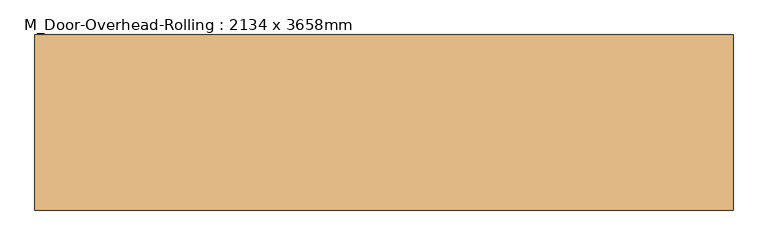
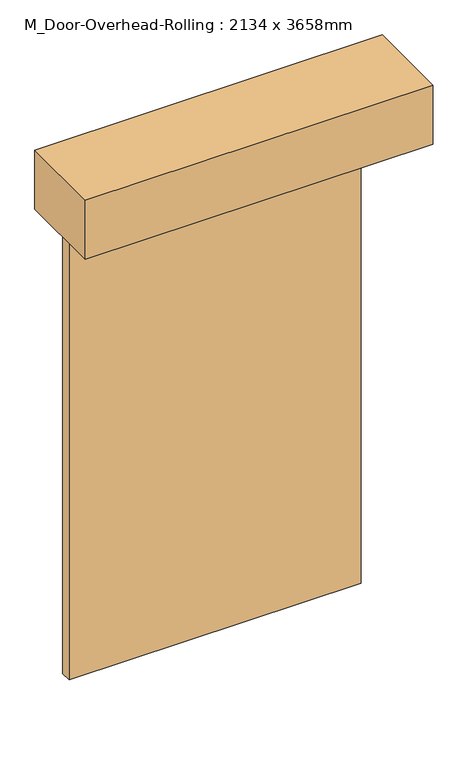
"""IFC4 building model written with IfcOpenShell, lengths in millimetres: door geometry, M_Door-Overhead-Rolling : 2134 x 3658mm."""

from ifc_helpers import new_model, si_unit, frame, origin, origin_with_axes, place, context, project, spatial, polyline, outline, extrude, source, transform, mapped, element, save


def m_door_overhead_rolling_2134_x_3658mm_be0fe279(model_context):
    return source(origin(), model_context, "Body", "SweptSolid", [
        extrude(outline(polyline([(1066.8, -114.3), (1066.8, -194.3), (-1066.8, -194.3), (-1066.8, -114.3), (1066.8, -114.3)])), origin_with_axes(), (0.0, 0.0, 1.0), 3657.6),
        extrude(outline(polyline([(1270.0, -753.1), (-1270.0, -753.1), (-1270.0, -114.3), (1270.0, -114.3), (1270.0, -753.1)])), frame((0.0, 0.0, 3657.6), z_axis=(0.0, 0.0, 1.0), x_axis=(1.0, 0.0, 0.0)), (0.0, 0.0, 1.0), 457.2),
    ])


if __name__ == "__main__":
    model = new_model("IFC4")
    model_context = context("Model", 3, world=origin())
    ifc_project = project(units=[si_unit("LENGTHUNIT", "METRE", prefix="MILLI")], contexts=[model_context])
    site = spatial("IfcSite", under=ifc_project)
    building = spatial("IfcBuilding", under=site)
    placement = place(None, origin())
    m_door_overhead_rolling_2134_x_3658mm_shape = m_door_overhead_rolling_2134_x_3658mm_be0fe279(model_context)
    element("IfcDoor", 1, ObjectType="M_Door-Overhead-Rolling : 2134 x 3658mm", at=placement, inside=building, context=model_context, shape_type="MappedRepresentation", body=[
        mapped(m_door_overhead_rolling_2134_x_3658mm_shape, transform((0.0, 0.0, 0.0), x_axis=(1.0, 0.0, 0.0), y_axis=(0.0, 1.0, 0.0), z_axis=(0.0, 0.0, 1.0))),
    ])
    save(model, "model.ifc")

# Revit data of these elements
# Type "M_Door-Overhead-Rolling : 2134 x 3658mm"
#   Type Mark = "8"
#   Construction Type Id = "MDOOR"
#   Assembly Code = "B2030400"
#   Analytic Construction = "Metal"
#   Thickness = 0' - 3.14961"
#   Rough Width [instance default] = 13' - 9.35433"
#   Rough Height [instance default] = 13' - 9.35433"
#   Heat Transfer Coefficient (U) = 0.651978 BTU/(h·ft²·°F)
#   Height [instance default] = 13' - 9.35433"
#   Width [instance default] = 13' - 9.35433"
#   Define Thermal Properties by = 1
#   Function = 1
#   Roller Material = Steel, Paint Finish, Ivory, Matte
#   Roller Box Material = Steel, Paint Finish, Ivory, Matte
#   Visual Light Transmittance = 0
#   Solar Heat Gain Coefficient = 0
#   Wall Closure = (empty or 0)
# Element 1 (IfcDoor, "M_Door-Overhead-Rolling : 2134 x 3658mm")
#   Rough Width = 7' - 0"
#   Rough Height = 12' - 0"
#   Height = 12' - 0"
#   Width = 7' - 0"
#   Materials on its faces: "Steel, Paint Finish, Ivory, Matte"
# Materials
#   "Steel, Paint Finish, Ivory, Matte": class "Metal", colour RGB 247 247 239, transparency 0, Description = "Steel, paint finish, ivory, matte", Cost = 0
